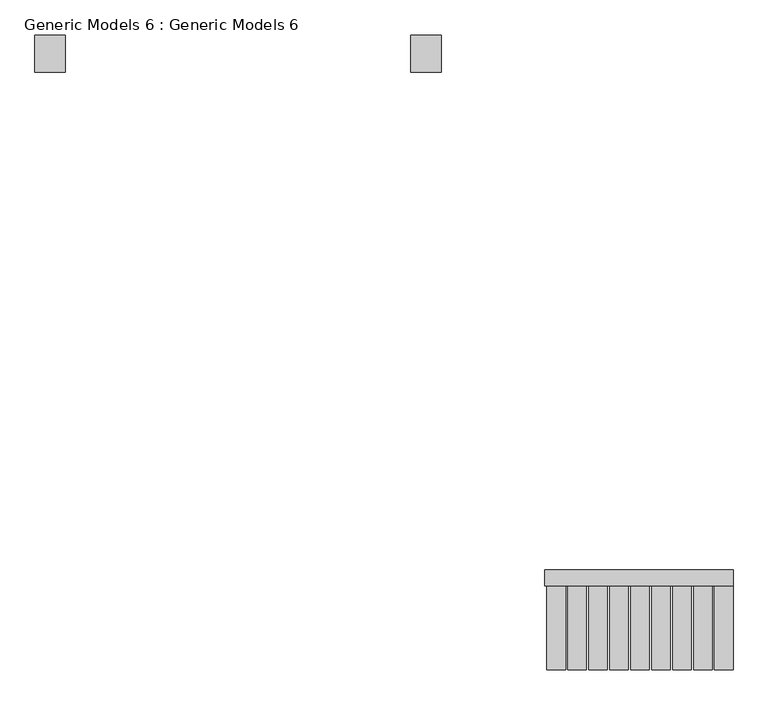
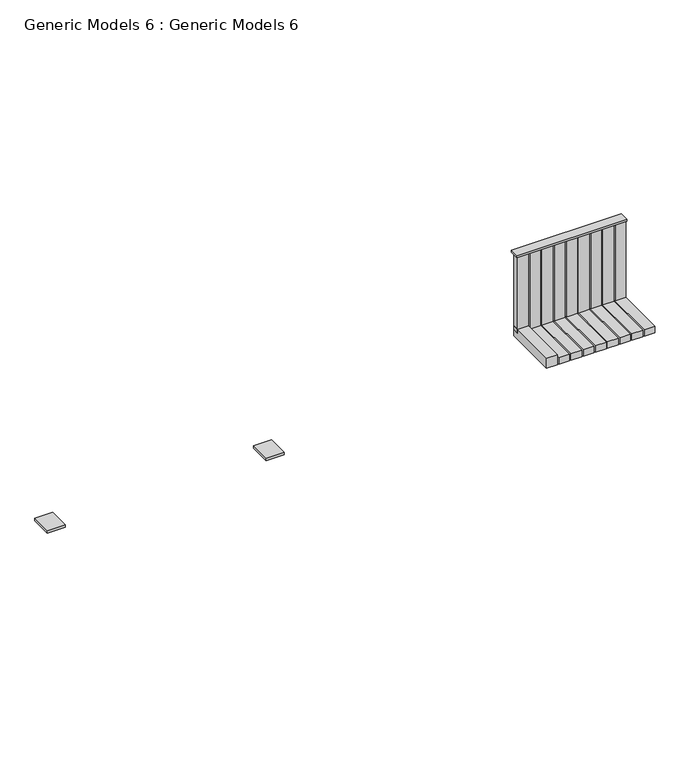
"""IFC4 building model written with IfcOpenShell, lengths in millimetres: proxy geometry, Generic Models 6 : Generic Models 6."""

from ifc_helpers import new_model, si_unit, frame, origin, place, context, project, spatial, polyline, outline, extrude, source, transform, mapped, element, save


def generic_models_6_generic_models_6_807765a8(model_context):
    return source(origin(), model_context, "Body", "SweptSolid", [
        extrude(outline(polyline([(-15329.468705, -5612.3027976), (-15659.668705, -5612.3027976), (-15659.668705, -5205.9027976), (-15329.468705, -5205.9027976), (-15329.468705, -5612.3027976)])), frame((0.0, 0.0, 2379.4594115), z_axis=(0.0, 0.0, 1.0), x_axis=(1.0, 0.0, 0.0)), (0.0, 0.0, 1.0), 50.8),
        extrude(outline(polyline([(-19431.568705, -5612.3027976), (-19761.768705, -5612.3027976), (-19761.768705, -5205.9027976), (-19431.568705, -5205.9027976), (-19431.568705, -5612.3027976)])), frame((0.0, 0.0, 2379.4594115), z_axis=(0.0, 0.0, 1.0), x_axis=(1.0, 0.0, 0.0)), (0.0, 0.0, 1.0), 50.8),
        extrude(outline(polyline([(-14199.168705, -11225.4395107), (-14199.168705, -11047.9027976), (-12141.768705, -11047.9027976), (-12141.768705, -11225.4395107), (-14199.168705, -11225.4395107)])), frame((0.0, 0.0, 9296.4), z_axis=(0.0, 0.0, 1.0), x_axis=(1.0, 0.0, 0.0)), (0.0, 0.0, 1.0), 38.1),
        extrude(outline(polyline([(-12344.968705, -11073.3027976), (-12141.768705, -11073.3027976), (-12141.768705, -11200.0395107), (-12344.968705, -11200.0395107), (-12344.968705, -11073.3027976)])), frame((0.0, 0.0, 7772.4), z_axis=(0.0, 0.0, 1.0), x_axis=(1.0, 0.0, 0.0)), (0.0, 0.0, 1.0), 1524.0),
        extrude(outline(polyline([(-12573.568705, -11073.3027976), (-12370.368705, -11073.3027976), (-12370.368705, -11200.0395107), (-12573.568705, -11200.0395107), (-12573.568705, -11073.3027976)])), frame((0.0, 0.0, 7772.4), z_axis=(0.0, 0.0, 1.0), x_axis=(1.0, 0.0, 0.0)), (0.0, 0.0, 1.0), 1524.0),
        extrude(outline(polyline([(-12802.168705, -11073.3027976), (-12598.968705, -11073.3027976), (-12598.968705, -11200.0395107), (-12802.168705, -11200.0395107), (-12802.168705, -11073.3027976)])), frame((0.0, 0.0, 7772.4), z_axis=(0.0, 0.0, 1.0), x_axis=(1.0, 0.0, 0.0)), (0.0, 0.0, 1.0), 1524.0),
        extrude(outline(polyline([(-13030.768705, -11073.3027976), (-12827.568705, -11073.3027976), (-12827.568705, -11200.0395107), (-13030.768705, -11200.0395107), (-13030.768705, -11073.3027976)])), frame((0.0, 0.0, 7772.4), z_axis=(0.0, 0.0, 1.0), x_axis=(1.0, 0.0, 0.0)), (0.0, 0.0, 1.0), 1524.0),
        extrude(outline(polyline([(-13259.368705, -11073.3027976), (-13056.168705, -11073.3027976), (-13056.168705, -11200.0395107), (-13259.368705, -11200.0395107), (-13259.368705, -11073.3027976)])), frame((0.0, 0.0, 7772.4), z_axis=(0.0, 0.0, 1.0), x_axis=(1.0, 0.0, 0.0)), (0.0, 0.0, 1.0), 1524.0),
        extrude(outline(polyline([(-13487.968705, -11073.3027976), (-13284.768705, -11073.3027976), (-13284.768705, -11200.0395107), (-13487.968705, -11200.0395107), (-13487.968705, -11073.3027976)])), frame((0.0, 0.0, 7772.4), z_axis=(0.0, 0.0, 1.0), x_axis=(1.0, 0.0, 0.0)), (0.0, 0.0, 1.0), 1524.0),
        extrude(outline(polyline([(-13716.568705, -11073.3027976), (-13513.368705, -11073.3027976), (-13513.368705, -11200.0395107), (-13716.568705, -11200.0395107), (-13716.568705, -11073.3027976)])), frame((0.0, 0.0, 7772.4), z_axis=(0.0, 0.0, 1.0), x_axis=(1.0, 0.0, 0.0)), (0.0, 0.0, 1.0), 1524.0),
        extrude(outline(polyline([(-13945.168705, -11073.3027976), (-13741.968705, -11073.3027976), (-13741.968705, -11200.0395107), (-13945.168705, -11200.0395107), (-13945.168705, -11073.3027976)])), frame((0.0, 0.0, 7772.4), z_axis=(0.0, 0.0, 1.0), x_axis=(1.0, 0.0, 0.0)), (0.0, 0.0, 1.0), 1524.0),
        extrude(outline(polyline([(-14173.768705, -11073.3027976), (-13970.568705, -11073.3027976), (-13970.568705, -11200.0395107), (-14173.768705, -11200.0395107), (-14173.768705, -11073.3027976)])), frame((0.0, 0.0, 7772.4), z_axis=(0.0, 0.0, 1.0), x_axis=(1.0, 0.0, 0.0)), (0.0, 0.0, 1.0), 1524.0),
        extrude(outline(polyline([(-12344.968705, -11073.3027976), (-12141.768705, -11073.3027976), (-12141.768705, -12140.1027976), (-12344.968705, -12140.1027976), (-12344.968705, -11073.3027976)])), frame((0.0, 0.0, 7645.4), z_axis=(0.0, 0.0, 1.0), x_axis=(1.0, 0.0, 0.0)), (0.0, 0.0, 1.0), 127.0),
        extrude(outline(polyline([(-12573.568705, -11073.3027976), (-12370.368705, -11073.3027976), (-12370.368705, -12140.1027976), (-12573.568705, -12140.1027976), (-12573.568705, -11073.3027976)])), frame((0.0, 0.0, 7645.4), z_axis=(0.0, 0.0, 1.0), x_axis=(1.0, 0.0, 0.0)), (0.0, 0.0, 1.0), 127.0),
        extrude(outline(polyline([(-12802.168705, -11073.3027976), (-12598.968705, -11073.3027976), (-12598.968705, -12140.1027976), (-12802.168705, -12140.1027976), (-12802.168705, -11073.3027976)])), frame((0.0, 0.0, 7645.4), z_axis=(0.0, 0.0, 1.0), x_axis=(1.0, 0.0, 0.0)), (0.0, 0.0, 1.0), 127.0),
        extrude(outline(polyline([(-13030.768705, -11073.3027976), (-12827.568705, -11073.3027976), (-12827.568705, -12140.1027976), (-13030.768705, -12140.1027976), (-13030.768705, -11073.3027976)])), frame((0.0, 0.0, 7645.4), z_axis=(0.0, 0.0, 1.0), x_axis=(1.0, 0.0, 0.0)), (0.0, 0.0, 1.0), 127.0),
        extrude(outline(polyline([(-13259.368705, -11073.3027976), (-13056.168705, -11073.3027976), (-13056.168705, -12140.1027976), (-13259.368705, -12140.1027976), (-13259.368705, -11073.3027976)])), frame((0.0, 0.0, 7645.4), z_axis=(0.0, 0.0, 1.0), x_axis=(1.0, 0.0, 0.0)), (0.0, 0.0, 1.0), 127.0),
        extrude(outline(polyline([(-13487.968705, -11073.3027976), (-13284.768705, -11073.3027976), (-13284.768705, -12140.1027976), (-13487.968705, -12140.1027976), (-13487.968705, -11073.3027976)])), frame((0.0, 0.0, 7645.4), z_axis=(0.0, 0.0, 1.0), x_axis=(1.0, 0.0, 0.0)), (0.0, 0.0, 1.0), 127.0),
        extrude(outline(polyline([(-13716.568705, -11073.3027976), (-13513.368705, -11073.3027976), (-13513.368705, -12140.1027976), (-13716.568705, -12140.1027976), (-13716.568705, -11073.3027976)])), frame((0.0, 0.0, 7645.4), z_axis=(0.0, 0.0, 1.0), x_axis=(1.0, 0.0, 0.0)), (0.0, 0.0, 1.0), 127.0),
        extrude(outline(polyline([(-13945.168705, -11073.3027976), (-13741.968705, -11073.3027976), (-13741.968705, -12140.1027976), (-13945.168705, -12140.1027976), (-13945.168705, -11073.3027976)])), frame((0.0, 0.0, 7645.4), z_axis=(0.0, 0.0, 1.0), x_axis=(1.0, 0.0, 0.0)), (0.0, 0.0, 1.0), 127.0),
        extrude(outline(polyline([(-14173.768705, -11073.3027976), (-13970.568705, -11073.3027976), (-13970.568705, -12140.1027976), (-14173.768705, -12140.1027976), (-14173.768705, -11073.3027976)])), frame((0.0, 0.0, 7645.4), z_axis=(0.0, 0.0, 1.0), x_axis=(1.0, 0.0, 0.0)), (0.0, 0.0, 1.0), 203.2),
    ])


if __name__ == "__main__":
    model = new_model("IFC4")
    model_context = context("Model", 3, world=origin())
    ifc_project = project(units=[si_unit("LENGTHUNIT", "METRE", prefix="MILLI")], contexts=[model_context])
    site = spatial("IfcSite", under=ifc_project)
    building = spatial("IfcBuilding", under=site)
    placement = place(None, origin())
    generic_models_6_generic_models_6_shape = generic_models_6_generic_models_6_807765a8(model_context)
    element("IfcBuildingElementProxy", 1, Name="Generic Models 6 : Generic Models 6", ObjectType="Generic Models 6 : Generic Models 6", at=placement, inside=building, context=model_context, shape_type="MappedRepresentation", body=[
        mapped(generic_models_6_generic_models_6_shape, transform((0.0, 0.0, 0.0), x_axis=(1.0, 0.0, 0.0), y_axis=(0.0, 1.0, 0.0), z_axis=(0.0, 0.0, 1.0))),
    ])
    save(model, "model.ifc")

# Revit data of these elements
# Element 1 (IfcBuildingElementProxy, "Generic Models 6 : Generic Models 6")
#   Materials on its faces: "Wood Planks"
# Materials
#   "Wood Planks": class "Wood", colour RGB 129 72 39, transparency 0, Description = "Physical material.", Cost = 0
